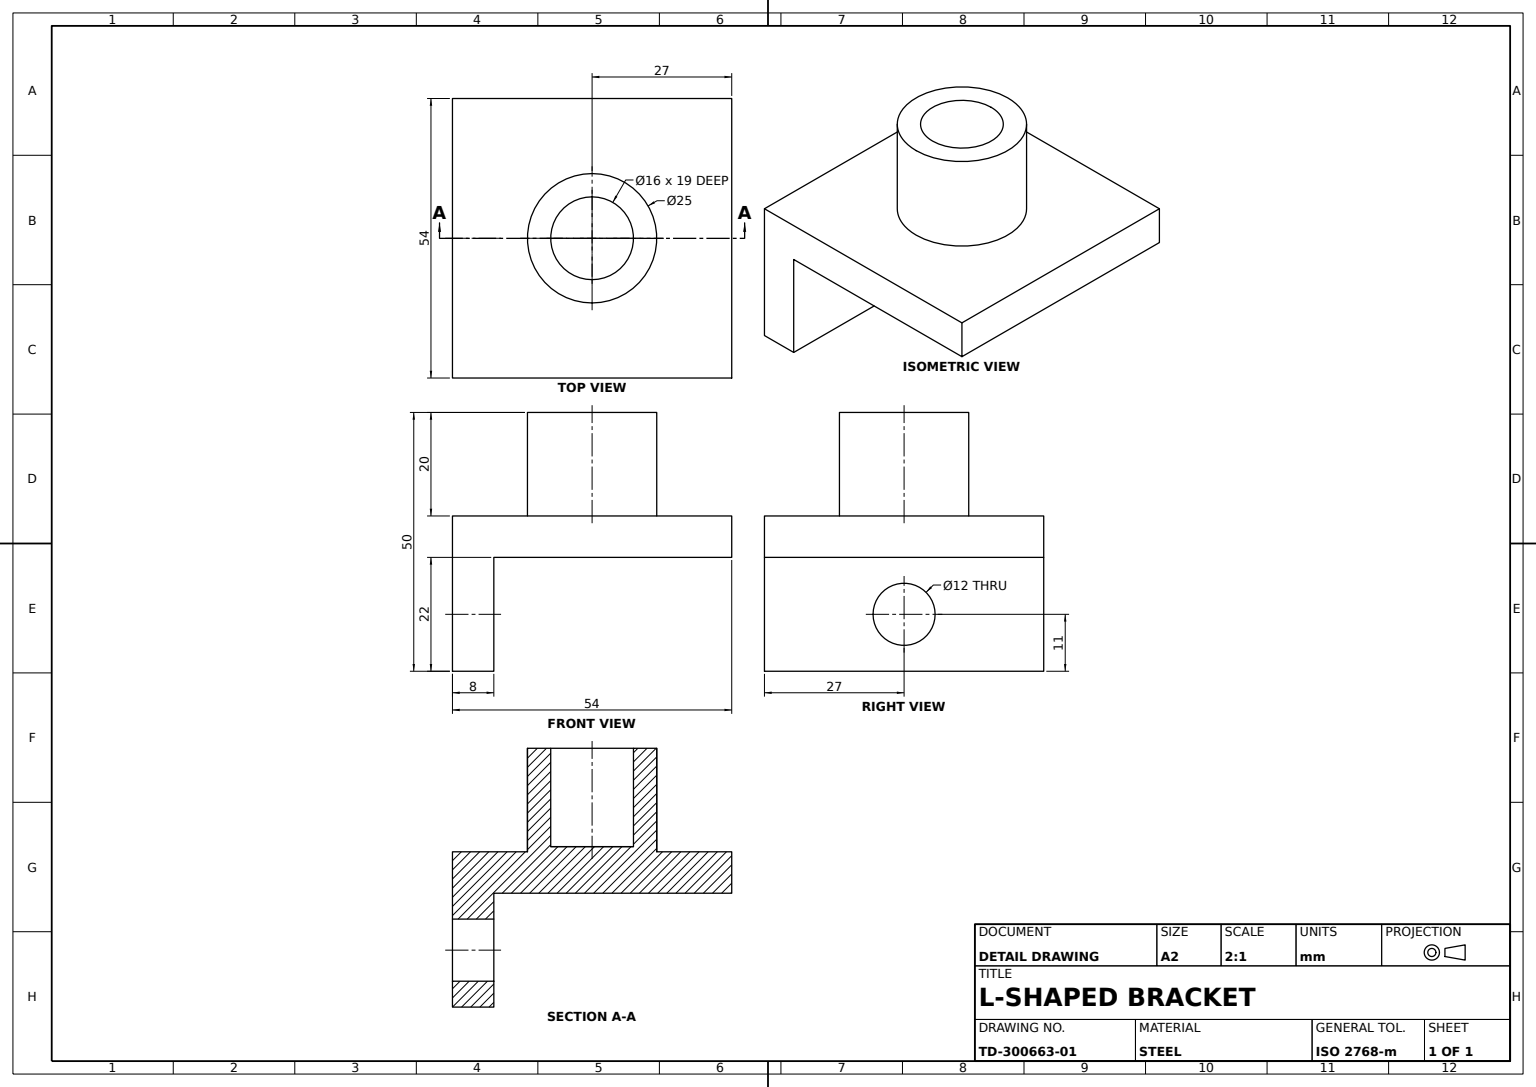
from build123d import *

# Parameters (mm, degrees)
BRACKET_BODY_DEPTH = 54
BOSS_SKETCH_R      = 12.5
BOSS_25_DEPTH      = 20
BORE_SKETCH_R      = 8
BORE_16_DEPTH      = 19
HOLE_SKETCH_R      = 6
HOLE_12_DEPTH      = 8


with BuildPart() as part:
    # Bracket Profile Sketch → Bracket Body (new body)
    with BuildSketch(Plane.XY):
        Polygon((0, 0), (0, 30), (54, 30), (54, 22), (8, 22), (8, 0), align=None)
    extrude(amount=BRACKET_BODY_DEPTH)

    # Boss Sketch → Boss Ø25 (add)
    with BuildSketch(Plane(origin=(0, 30, 0), x_dir=(1, 0, 0), z_dir=(0, 1, 0))):
        with Locations(Location((27, -27, 0), (0, 0, 270))):
            Circle(BOSS_SKETCH_R)
    extrude(amount=BOSS_25_DEPTH)

    # Bore Sketch → Bore Ø16 (cut)
    with BuildSketch(Plane(origin=(0, 50, 0), x_dir=(1, 0, 0), z_dir=(0, 1, 0))):
        with Locations(Location((27, -27, 0), (0, 0, 270))):
            Circle(BORE_SKETCH_R)
    extrude(amount=-BORE_16_DEPTH, mode=Mode.SUBTRACT)

    # Hole Sketch → Hole Ø12 (cut)
    with BuildSketch(Plane(origin=(8, 0, 0), x_dir=(0, 0, -1), z_dir=(1, 0, 0))):
        with Locations((-27, 11)):
            Circle(HOLE_SKETCH_R)
    extrude(amount=-HOLE_12_DEPTH, mode=Mode.SUBTRACT)


solid = part.part
